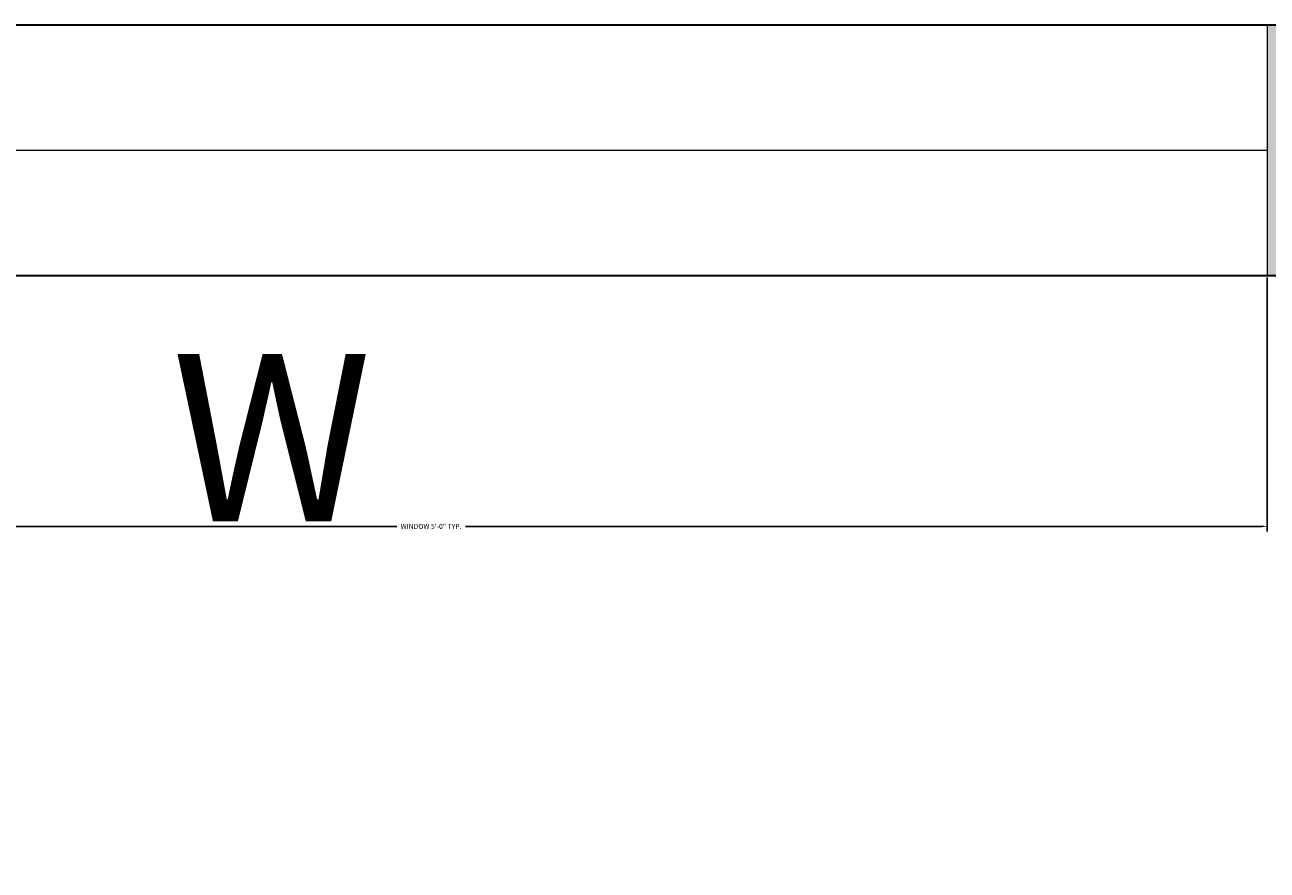
# Model space of a CAD drawing. Units: inches. Extents: x -5 to 330, y -522 to 40.
# Tile 15 of 23: x 201 to 246, y -447 to -417. Entities that reach past the tile are written whole.
import ezdxf

# ---------------------------------------------------------------- set-up
doc = ezdxf.new("R2010")
doc.units = ezdxf.units.IN
doc.header["$MEASUREMENT"] = 0
for name, color, linetype, lineweight in [('A-ANNO-DIMS', 2, 'Continuous', 18), ('A-ANNO-TEXT', 7, 'Continuous', 18), ('A-GLAZ', 4, 'Continuous', 18), ('A-WALL', 7, 'Continuous', 35)]:
    doc.layers.add(name, color=color, linetype=linetype, lineweight=lineweight)
doc.layers.add('A-WALL-PATT', color=18, linetype='Continuous', lineweight=13, true_color=0x000000)
doc.styles.get("Standard").update_dxf_attribs({"font": 'arial.ttf'})
doc.dimstyles.get("Standard").update_dxf_attribs({"dimtxt": 0.18, "dimasz": 0.18, "dimexe": 0.18, "dimexo": 0.0625, "dimgap": 0.09, "dimtad": 0, "dimtih": 1, "dimtoh": 1, "dimdec": 0, "dimzin": 0, "dimdsep": 46, "dimlunit": 3, "dimtxsty": 'Standard', "dimcen": 0.09, "dimadec": 0, "dimazin": 0, "dimtfac": 1, "dimtdec": 0, "dimtofl": 0, "dimtmove": 0, "dimatfit": 3, "dimfxl": 1, "dimtolj": 1, "dimtzin": 0, "dimarcsym": 0})

# ---------------------------------------------------------------- blocks, each defined once
blk = doc.blocks.new('WIN-60IN-GLAZ')
for p, q in [((0, 9), (60, 9)), ((0, 4.5), (60, 4.5)), ((60, 0), (0, 0))]:
    blk.add_line(p, q)
blk = doc.blocks.new('*D19')
at = {"layer": 'A-ANNO-DIMS', "color": 0, "lineweight": -2, "transparency": 16777216}
for p, q in [((185.51, -426.206), (185.51, -435.324)), ((245.51, -426.206), (245.51, -435.324)), ((185.69, -435.144), (214.281, -435.144)), ((245.33, -435.144), (216.739, -435.144))]:
    blk.add_line(p, q, dxfattribs=at)
at = {"layer": 'A-ANNO-DIMS', "color": 0, "transparency": 16777216}
for points in [[(185.69, -435.114), (185.69, -435.174), (185.51, -435.144)], [(245.33, -435.114), (245.33, -435.174), (245.51, -435.144)]]:
    blk.add_solid(points, dxfattribs=at)
at = {"layer": 'Defpoints', "color": 0, "transparency": 16777216}
for p in [(185.51, -426.144), (245.51, -426.144), (245.51, -435.144)]:
    blk.add_point(p, dxfattribs=at)
at = {"layer": 'A-ANNO-DIMS', "color": 0, "transparency": 16777216, "insert": (215.51, -435.144), "char_height": 0.18, "attachment_point": 5}
blk.add_mtext('\\A1;WINDOW 5\'-0" TYP.', dxfattribs=at)
blk = doc.blocks.new('*D20')
at = {"layer": 'A-ANNO-DIMS', "color": 0, "lineweight": -2, "transparency": 16777216}
for p, q in [((245.572, -417.144), (254.69, -417.144)), ((254.51, -417.324), (254.51, -421.462)), ((254.51, -425.964), (254.51, -421.825)), ((245.572, -426.144), (254.69, -426.144))]:
    blk.add_line(p, q, dxfattribs=at)
at = {"layer": 'A-ANNO-DIMS', "color": 0, "transparency": 16777216}
for points in [[(254.48, -417.324), (254.54, -417.324), (254.51, -417.144)], [(254.48, -425.964), (254.54, -425.964), (254.51, -426.144)]]:
    blk.add_solid(points, dxfattribs=at)
at = {"layer": 'Defpoints', "color": 0, "transparency": 16777216}
for p in [(245.51, -417.144), (254.51, -417.144), (245.51, -426.144)]:
    blk.add_point(p, dxfattribs=at)
at = {"layer": 'A-ANNO-DIMS', "color": 0, "transparency": 16777216, "insert": (254.51, -421.644), "char_height": 0.18, "attachment_point": 5}
blk.add_mtext('\\A1;0\'-9" TYP.', dxfattribs=at)
blk = doc.blocks.new('*D37')
at = {"layer": 'A-ANNO-DIMS', "color": 0, "lineweight": -2, "transparency": 16777216}
for p, q in [((164.01, -53.206), (164.01, -522.309)), ((272.01, -53.206), (272.01, -522.309)), ((164.19, -522.129), (217.681, -522.129)), ((271.83, -522.129), (218.339, -522.129))]:
    blk.add_line(p, q, dxfattribs=at)
at = {"layer": 'A-ANNO-DIMS', "color": 0, "transparency": 16777216}
for points in [[(164.19, -522.099), (164.19, -522.159), (164.01, -522.129)], [(271.83, -522.099), (271.83, -522.159), (272.01, -522.129)]]:
    blk.add_solid(points, dxfattribs=at)
at = {"layer": 'Defpoints', "color": 0, "transparency": 16777216}
for p in [(164.01, -53.144), (272.01, -53.144), (272.01, -522.129)]:
    blk.add_point(p, dxfattribs=at)
at = {"layer": 'A-ANNO-DIMS', "color": 0, "transparency": 16777216, "insert": (218.01, -522.129), "char_height": 0.18, "attachment_point": 5}
blk.add_mtext('\\A1;9\'-0"', dxfattribs=at)

msp = doc.modelspace()

# ---------------------------------------------------------------- hatches: boundary and pattern name
at = {"layer": 'A-WALL-PATT'}
h = msp.add_hatch(color=256, dxfattribs=at)
h.dxf.hatch_style = 1
h.paths.add_polyline_path([(164.01, -44.152), (159.51, -44.152), (159.51, -153.144), (164.01, -153.144)], flags=17)
h.paths.add_polyline_path([(224.01, -188.144), (272.01, -188.144), (272.01, -218.144), (260.01, -218.144), (260.01, -222.644), (272.01, -222.644), (272.01, -292.644), (159.01, -292.644), (159.01, -297.144), (272.01, -297.144), (272.01, -417.144), (245.51, -417.144), (245.51, -426.144), (272.01, -426.144), (272.01, -495.144), (281.01, -495.144), (281.01, 12.356), (23.51, 12.356), (23.51, -426.144), (62.918, -426.144), (62.918, -417.144), (32.51, -417.144), (32.51, -297.144), (48.129, -297.144), (48.129, -292.644), (32.51, -292.644), (32.51, -140.644), (133.51, -140.644), (133.51, -131.644), (32.51, -131.644), (32.51, 3.356), (159.51, 3.356), (164.01, 3.356), (220.01, 3.356), (224.51, 3.356), (272.01, 3.356), (272.01, -179.144), (159.51, -179.144), (159.51, -188.144), (219.51, -188.144), (219.51, -266.644), (224.01, -266.644), (224.01, -222.644), (236.01, -222.644), (236.01, -218.144), (224.01, -218.144)])
h.paths.add_polyline_path([(133.01, -292.644), (128.51, -292.644), (128.51, -297.144), (128.51, -417.144), (122.918, -417.144), (122.918, -426.144), (133.01, -426.144)], flags=17)
h.paths.add_polyline_path([(185.51, -417.144), (159.01, -417.144), (159.01, -426.144), (185.51, -426.144)], flags=17)
h.paths.add_polyline_path([(133.51, -140.644), (129.01, -140.644), (129.01, -246.644), (133.51, -246.644)], flags=17)
h.paths.add_polyline_path([(246.01, -48.644), (224.51, -48.644), (224.51, -27.627), (220.01, -27.627), (220.01, -48.644), (198.604, -48.644), (198.604, -53.144), (246.01, -53.144)], flags=17)

# ---------------------------------------------------------------- linework, layer by layer
at = {"layer": 'A-GLAZ'}
msp.add_line((245.51, -417.144), (245.51, -426.144), dxfattribs=at)
at = {"layer": 'A-WALL'}
for p, q in [((159.01, -417.144), (272.01, -417.144)), ((159.01, -426.144), (272.01, -426.144))]:
    msp.add_line(p, q, dxfattribs=at)

# ---------------------------------------------------------------- block references
at = {"layer": 'A-GLAZ'}
msp.add_blockref('WIN-60IN-GLAZ', (185.51, -426.144), dxfattribs=at)

# ---------------------------------------------------------------- texts
at = {"layer": 'A-ANNO-TEXT', "insert": (206.197, -428.957), "char_height": 6, "attachment_point": 1}
msp.add_mtext('W', dxfattribs=at)

# ---------------------------------------------------------------- dimensions: what is measured, and where the dimension line sits
at = {"layer": 'A-ANNO-DIMS'}
dim = msp.add_linear_dim(base=(272.01, -522.129), p1=(164.01, -53.144), p2=(272.01, -53.144), dimstyle='Standard', override={"dimdec": 1, "dimlfac": 1, "dimrnd": 0, "dimzin": 1, "dimdsep": 46, "dimlunit": 4, "dimfrac": 2}, dxfattribs=at)
dim.commit()
dim.dimension.update_dxf_attribs({"geometry": '*D37', "text_midpoint": (218.01, -522.129)})
dim = msp.add_linear_dim(base=(254.51, -417.144), p1=(245.51, -426.144), p2=(245.51, -417.144), angle=90, text='<> TYP.', dimstyle='Standard', override={"dimdec": 1, "dimlfac": 1, "dimrnd": 0, "dimzin": 1, "dimdsep": 46, "dimlunit": 4, "dimfrac": 2}, dxfattribs=at)
dim.commit()
dim.dimension.update_dxf_attribs({"geometry": '*D20', "text_midpoint": (254.51, -421.644)})
dim = msp.add_linear_dim(base=(245.51, -435.144), p1=(185.51, -426.144), p2=(245.51, -426.144), text='WINDOW <> TYP.', dimstyle='Standard', override={"dimdec": 1, "dimlfac": 1, "dimrnd": 0, "dimzin": 1, "dimdsep": 46, "dimlunit": 4, "dimfrac": 2}, dxfattribs=at)
dim.commit()
dim.dimension.update_dxf_attribs({"geometry": '*D19', "text_midpoint": (215.51, -435.144)})

doc.saveas('drawing.dxf')
